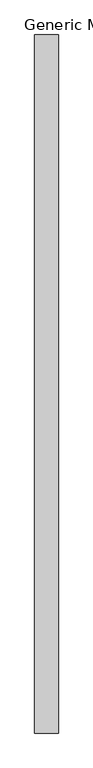
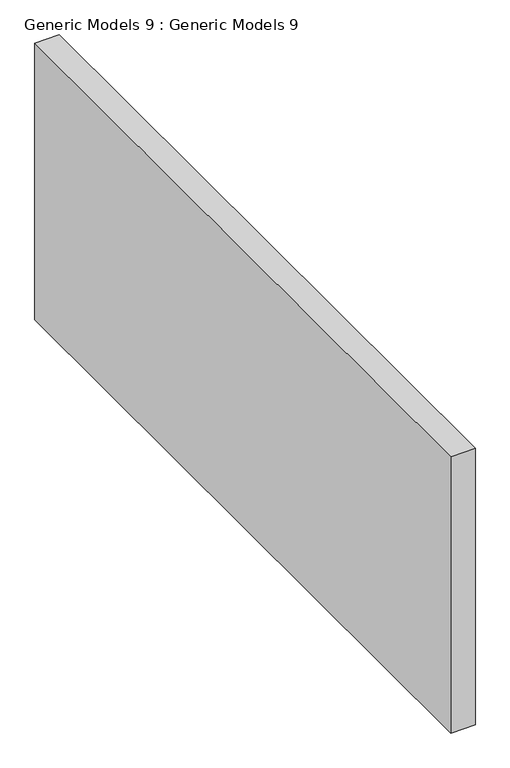
"""IFC4 building model written with IfcOpenShell, lengths in millimetres: proxy geometry, Generic Models 9 : Generic Models 9."""

from ifc_helpers import new_model, si_unit, frame, origin, place, context, project, spatial, polyline, outline, extrude, source, transform, mapped, element, save


def generic_models_9_generic_models_9_a63bbd8a(model_context):
    return source(origin(), model_context, "Body", "SweptSolid", [
        extrude(outline(polyline([(548.4218735, -4389.2142532), (548.4218735, -5887.8142532), (497.6218735, -5887.8142532), (497.6218735, -4389.2142532), (548.4218735, -4389.2142532)])), frame((0.0, 0.0, 5792.9831442), z_axis=(0.0, 0.0, 1.0), x_axis=(1.0, 0.0, 0.0)), (0.0, 0.0, 1.0), 607.8168558),
    ])


if __name__ == "__main__":
    model = new_model("IFC4")
    model_context = context("Model", 3, world=origin())
    ifc_project = project(units=[si_unit("LENGTHUNIT", "METRE", prefix="MILLI")], contexts=[model_context])
    site = spatial("IfcSite", under=ifc_project)
    building = spatial("IfcBuilding", under=site)
    placement = place(None, origin())
    generic_models_9_generic_models_9_shape = generic_models_9_generic_models_9_a63bbd8a(model_context)
    element("IfcBuildingElementProxy", 1, Name="Generic Models 9 : Generic Models 9", ObjectType="Generic Models 9 : Generic Models 9", at=placement, inside=building, context=model_context, shape_type="MappedRepresentation", body=[
        mapped(generic_models_9_generic_models_9_shape, transform((0.0, 0.0, 0.0), x_axis=(1.0, 0.0, 0.0), y_axis=(0.0, 1.0, 0.0), z_axis=(0.0, 0.0, 1.0))),
    ])
    save(model, "model.ifc")
